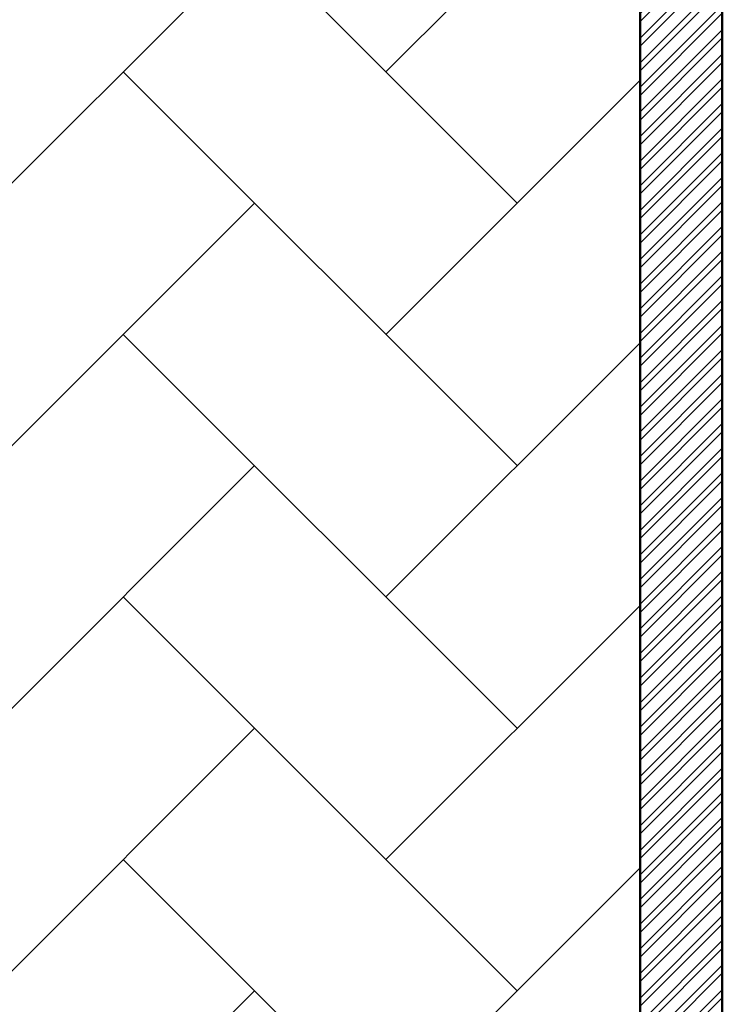
# Model space of a CAD drawing. Units: inches. Extents: x 3590 to 5167, y 65 to 1917.
# Tile 56 of 100: x 5003 to 5080, y 1450 to 1558. Entities that reach past the tile are written whole.
import ezdxf

# ---------------------------------------------------------------- set-up
doc = ezdxf.new("R2010")
doc.units = ezdxf.units.IN
for name, color, linetype, lineweight in [('A-FLOR-PATT', 8, 'Continuous', 13), ('A-WALL', 7, 'Continuous', 50), ('A-WALL-PATT', 251, 'Continuous', 13)]:
    doc.layers.add(name, color=color, linetype=linetype, lineweight=lineweight)

msp = doc.modelspace()

# ---------------------------------------------------------------- hatches: boundary and pattern name
at = {"layer": 'A-FLOR-PATT', "transparency": 33554687}
h = msp.add_hatch(dxfattribs=at)
h.set_pattern_fill('AR-HBONE', color=256, scale=0.2)
h.set_pattern_definition([(45, (-588.972, 0), (0, 28.73682), [60.96, -20.32]), (135, (-574.604, 14.368), (3e-15, 28.73682), [60.96, -20.32])])
h.paths.add_polyline_path([(5071.27, 1797), (4933.27, 1797), (4933.27, 1754), (4962.77, 1754, -0.414214), (4928.77, 1720), (4933.27, 1719), (4933.27, 1335), (5071.27, 1335)])
h.paths.add_polyline_path([(4951.78, 1521.08), (4951.72, 1521.04), (4951.56, 1520.9)], flags=16)
h.paths.add_polyline_path([(4952.27, 1521.38), (4952.2, 1521.37), (4952.2, 1521.36)], flags=0)
h.paths.add_polyline_path([(4967.05, 1529.73), (4965.23, 1528.69), (4963.41, 1527.71), (4961.76, 1526.85), (4963.59, 1527.45), (4964.04, 1527.48), (4962.98, 1527.25), (4961.76, 1526.85), (4959.79, 1525.83), (4958, 1524.89), (4956.24, 1523.93), (4954.5, 1522.92), (4954.13, 1522.68), (4953.36, 1522), (4953.37, 1522), (4953.61, 1522.06), (4955.11, 1522.76), (4956.92, 1523.43), (4958.68, 1523.92), (4960.36, 1524.2), (4961.94, 1524.29), (4964.17, 1524.11), (4965.96, 1523.31), (4963.86, 1522.98), (4965.19, 1522.5), (4963.37, 1522.5), (4961.55, 1522.49), (4959.76, 1522.46), (4958.3, 1522.42), (4957.97, 1522.39), (4956.31, 1522.23), (4954.72, 1522.07), (4953.25, 1521.9), (4953.53, 1521.62), (4954.33, 1521.38), (4956.24, 1521.23), (4958.04, 1520.93), (4959.68, 1520.48), (4961.16, 1519.9), (4963.11, 1518.8), (4964.39, 1517.33), (4962.97, 1517.73), (4964.56, 1516.66), (4965.41, 1515.71), (4963.51, 1516.32), (4961.68, 1517.01), (4959.93, 1517.74), (4958.28, 1518.53), (4956.73, 1519.34), (4955.3, 1520.17), (4954.67, 1520.57), (4954.51, 1520.63), (4955.66, 1519.32), (4956.7, 1517.98), (4957.64, 1516.65), (4958.49, 1515.33), (4959.55, 1513.52), (4960.44, 1511.77), (4958.84, 1513.62), (4957.45, 1515.32), (4955.82, 1517.46), (4956.67, 1515.45), (4957.11, 1513.92), (4957.45, 1511.71), (4957.08, 1509.79), (4956.54, 1511.11), (4955.99, 1512.57), (4955.44, 1514.13), (4954.9, 1515.74), (4954.36, 1517.36), (4953.82, 1518.94), (4953.3, 1520.45), (4953.06, 1521.12), (4952.97, 1521.15), (4952.95, 1521.09), (4952.73, 1520.2), (4953.37, 1518.02), (4953.76, 1516.37), (4954.05, 1514.77), (4954.26, 1513.22), (4954.47, 1511.13), (4954.5, 1510.4), (4954.41, 1511.76), (4954.26, 1513.22), (4954.05, 1514.77), (4953.76, 1516.37), (4953.37, 1518.02), (4952.88, 1519.7), (4952.72, 1520.14), (4952.53, 1519.06), (4952.37, 1517.79), (4952.22, 1516.31), (4952.05, 1514.6), (4951.83, 1512.63), (4951.56, 1510.36), (4951.2, 1512.17), (4950.85, 1514.34), (4950.99, 1516.38), (4951.66, 1518.29), (4952.59, 1520.48), (4952.36, 1521.13), (4951.86, 1520.33), (4950.84, 1518.91), (4949.78, 1517.59), (4948.92, 1516.62), (4948.11, 1515.26), (4947.09, 1513.55), (4945.89, 1511.61), (4946.33, 1513.4), (4946.56, 1514.25), (4945.53, 1513.33), (4944.58, 1512.53), (4946.02, 1514.51), (4947.2, 1516.05), (4947.89, 1517.31), (4949.31, 1518.76), (4950.41, 1519.77), (4950.45, 1519.81), (4952.27, 1521.38), (4951.64, 1521.49), (4950.4, 1521.18), (4948.04, 1520.36), (4946.12, 1519.45), (4944.57, 1518.47), (4943.35, 1517.44), (4942, 1515.92), (4941.66, 1515.27), (4942.81, 1516.99), (4944.57, 1518.47), (4946.12, 1519.45), (4948.04, 1520.36), (4950.4, 1521.18), (4951.64, 1521.49), (4949.65, 1521.87), (4948.6, 1521.76), (4947.13, 1521.57), (4945.42, 1521.35), (4943.45, 1521.1), (4941.18, 1520.86), (4942.86, 1521.61), (4943.87, 1522.03), (4942.95, 1521.91), (4941.41, 1521.49), (4939.54, 1520.67), (4938.97, 1520.23), (4940.73, 1521.3), (4942.95, 1521.91), (4943.7, 1522.01), (4945.89, 1522.7), (4947.56, 1522.71), (4948.92, 1522.57), (4951.13, 1522.18), (4950.97, 1522.3), (4948.13, 1523.01), (4946.03, 1523.71), (4944.23, 1524.52), (4942.71, 1525.46), (4941.44, 1526.54), (4940.43, 1527.76), (4939.65, 1529.14), (4941.42, 1528.12), (4943.15, 1527.13), (4944.84, 1526.17), (4946.51, 1525.25), (4948.18, 1524.36), (4948.36, 1524.26), (4946.48, 1526.04), (4945.18, 1527.54), (4944.19, 1529.03), (4943.5, 1530.54), (4943.28, 1531.36), (4942.5, 1531.92), (4943.11, 1531.76), (4942.96, 1533.66), (4944.14, 1531.99), (4944.61, 1531.32), (4946.2, 1530.46), (4947.49, 1529.51), (4948.79, 1528.23), (4950.37, 1526.24), (4949.49, 1528.16), (4948.85, 1530.12), (4948.49, 1532.04), (4948.38, 1533.92), (4948.5, 1535.76), (4948.83, 1537.57), (4949.42, 1535.57), (4949.96, 1533.57), (4950.46, 1531.59), (4950.96, 1529.62), (4951.39, 1527.95), (4951.72, 1530.69), (4952.2, 1532.58), (4952.89, 1534.33), (4953.77, 1535.95), (4954.83, 1537.46), (4954.52, 1535.39), (4954.27, 1533.94), (4955.58, 1535.66), (4956.75, 1536.74), (4956.16, 1534.78), (4955.59, 1532.87), (4955.04, 1531.01), (4954.52, 1529.17), (4954.04, 1527.34), (4953.64, 1525.73), (4953.61, 1525.59), (4953.4, 1524.17), (4953.38, 1524.01), (4954.07, 1525.48), (4954.91, 1527.02), (4956.14, 1528.89), (4957.85, 1530.58), (4959.38, 1531.54), (4958.26, 1530.1), (4957.14, 1528.66), (4956.07, 1527.24), (4955.06, 1525.87), (4954.14, 1524.57), (4953.35, 1523.37), (4953.31, 1523.3), (4953.27, 1522.92), (4953.26, 1522.38), (4954.1, 1523.37), (4954.63, 1524.28), (4955.96, 1526.36), (4957.23, 1528.13), (4958.42, 1529.61), (4960.04, 1531.37), (4961.37, 1532.38), (4962.1, 1532.77), (4961.07, 1531.06), (4959.99, 1529.44), (4958.87, 1527.91), (4958.15, 1527.01), (4959.8, 1528), (4961.59, 1528.79), (4963.39, 1529.33), (4965.21, 1529.63)], flags=16)
h.paths.add_polyline_path([(4962.94, 1523.18), (4961.11, 1523.42), (4960.39, 1523.36), (4962.35, 1523.33)], flags=0)
h.paths.add_polyline_path([(5049.54, 1584.55), (5049.48, 1584.51), (5049.32, 1584.37)], flags=16)
h.paths.add_polyline_path([(5050.03, 1584.85), (5049.96, 1584.85), (5049.96, 1584.83)], flags=0)
h.paths.add_polyline_path([(5042.33, 1581.95), (5043.88, 1582.93), (5045.81, 1583.83), (5048.16, 1584.65), (5049.41, 1584.97), (5047.41, 1585.34), (5046.36, 1585.23), (5044.89, 1585.04), (5043.18, 1584.82), (5041.21, 1584.58), (5038.94, 1584.33), (5040.62, 1585.09), (5041.63, 1585.5), (5040.71, 1585.38), (5039.17, 1584.96), (5037.3, 1584.14), (5036.73, 1583.7), (5038.49, 1584.77), (5040.71, 1585.38), (5041.46, 1585.48), (5043.66, 1586.17), (5045.33, 1586.19), (5046.68, 1586.04), (5048.89, 1585.66), (5048.73, 1585.77), (5045.89, 1586.48), (5043.8, 1587.18), (5041.99, 1588), (5040.47, 1588.94), (5039.21, 1590.01), (5038.19, 1591.23), (5037.41, 1592.62), (5039.18, 1591.6), (5040.91, 1590.61), (5042.6, 1589.65), (5044.28, 1588.72), (5045.94, 1587.83), (5046.13, 1587.74), (5044.24, 1589.52), (5042.94, 1591.01), (5041.95, 1592.51), (5041.26, 1594.01), (5041.04, 1594.83), (5040.26, 1595.39), (5040.87, 1595.24), (5040.72, 1597.13), (5041.9, 1595.46), (5042.37, 1594.8), (5043.96, 1593.94), (5045.25, 1592.98), (5046.55, 1591.7), (5048.13, 1589.71), (5047.25, 1591.63), (5046.61, 1593.6), (5046.25, 1595.52), (5046.14, 1597.39), (5046.26, 1599.23), (5046.59, 1601.05), (5047.18, 1599.04), (5047.72, 1597.04), (5048.23, 1595.06), (5048.72, 1593.09), (5049.15, 1591.43), (5049.48, 1594.16), (5049.96, 1596.05), (5050.65, 1597.8), (5051.53, 1599.43), (5052.59, 1600.93), (5052.28, 1598.86), (5052.03, 1597.41), (5053.34, 1599.14), (5054.51, 1600.21), (5053.92, 1598.25), (5053.35, 1596.35), (5052.8, 1594.48), (5052.29, 1592.64), (5051.8, 1590.82), (5051.4, 1589.21), (5051.37, 1589.06), (5051.16, 1587.64), (5051.14, 1587.48), (5051.83, 1588.95), (5052.67, 1590.5), (5053.9, 1592.37), (5055.61, 1594.05), (5057.14, 1595.01), (5056.02, 1593.58), (5054.9, 1592.14), (5053.83, 1590.72), (5052.82, 1589.34), (5051.9, 1588.05), (5051.11, 1586.85), (5051.07, 1586.78), (5051.03, 1586.4), (5051.02, 1585.86), (5051.86, 1586.85), (5052.39, 1587.76), (5053.72, 1589.83), (5054.99, 1591.6), (5056.18, 1593.08), (5057.8, 1594.84), (5059.13, 1595.85), (5059.86, 1596.24), (5058.83, 1594.54), (5057.75, 1592.91), (5056.63, 1591.38), (5055.91, 1590.48), (5057.56, 1591.48), (5059.35, 1592.27), (5061.15, 1592.8), (5062.97, 1593.11), (5064.81, 1593.2), (5062.99, 1592.17), (5061.17, 1591.19), (5059.52, 1590.32), (5061.35, 1590.92), (5061.8, 1590.95), (5060.74, 1590.72), (5059.52, 1590.33), (5057.55, 1589.31), (5055.77, 1588.37), (5054, 1587.4), (5052.27, 1586.39), (5051.89, 1586.16), (5051.12, 1585.47), (5051.13, 1585.47), (5051.37, 1585.54), (5052.87, 1586.24), (5054.68, 1586.91), (5056.44, 1587.39), (5058.12, 1587.67), (5059.71, 1587.76), (5061.93, 1587.58), (5063.72, 1586.78), (5061.62, 1586.45), (5062.95, 1585.97), (5061.13, 1585.97), (5059.31, 1585.96), (5057.52, 1585.93), (5056.07, 1585.89), (5055.73, 1585.86), (5054.07, 1585.71), (5052.48, 1585.55), (5051.01, 1585.37), (5051.29, 1585.1), (5052.09, 1584.85), (5054, 1584.7), (5055.8, 1584.4), (5057.45, 1583.96), (5058.92, 1583.37), (5060.87, 1582.27), (5062.15, 1580.8), (5060.73, 1581.2), (5062.32, 1580.13), (5063.17, 1579.18), (5061.27, 1579.8), (5059.44, 1580.48), (5057.7, 1581.22), (5056.04, 1582), (5054.49, 1582.82), (5053.06, 1583.65), (5052.43, 1584.05), (5052.27, 1584.1), (5053.42, 1582.79), (5054.46, 1581.46), (5055.41, 1580.12), (5056.25, 1578.81), (5057.31, 1577), (5058.2, 1575.24), (5056.6, 1577.09), (5055.21, 1578.8), (5053.58, 1580.93), (5054.43, 1578.92), (5054.87, 1577.4), (5055.21, 1575.19), (5054.84, 1573.27), (5054.3, 1574.58), (5053.75, 1576.04), (5053.21, 1577.6), (5052.66, 1579.21), (5052.12, 1580.83), (5051.59, 1582.42), (5051.07, 1583.93), (5050.83, 1584.59), (5050.73, 1584.62), (5050.71, 1584.56), (5050.49, 1583.67), (5051.13, 1581.5), (5051.52, 1579.85), (5051.81, 1578.24), (5052.03, 1576.7), (5052.23, 1574.61), (5052.26, 1573.88), (5052.17, 1575.23), (5052.03, 1576.7), (5051.81, 1578.24), (5051.52, 1579.85), (5051.13, 1581.5), (5050.64, 1583.17), (5050.48, 1583.62), (5050.29, 1582.53), (5050.14, 1581.26), (5049.98, 1579.79), (5049.81, 1578.07), (5049.59, 1576.1), (5049.32, 1573.84), (5048.96, 1575.64), (5048.61, 1577.81), (5048.75, 1579.85), (5049.42, 1581.76), (5050.35, 1583.96), (5050.12, 1584.6), (5049.62, 1583.8), (5048.6, 1582.38), (5047.54, 1581.06), (5046.68, 1580.09), (5045.87, 1578.73), (5044.85, 1577.03), (5043.65, 1575.09), (5044.09, 1576.88), (5044.32, 1577.72), (5043.29, 1576.8), (5042.34, 1576.01), (5043.78, 1577.98), (5044.97, 1579.52), (5045.65, 1580.79), (5047.07, 1582.24), (5048.18, 1583.24), (5048.21, 1583.28), (5050.03, 1584.85), (5049.41, 1584.97), (5048.16, 1584.65), (5045.81, 1583.83), (5043.88, 1582.93), (5042.33, 1581.95), (5041.11, 1580.92), (5039.76, 1579.39), (5039.42, 1578.75), (5040.57, 1580.46)], flags=16)
h.paths.add_polyline_path([(4954.8, 1533.12), (4954.26, 1532.08), (4953.83, 1530.93), (4953.5, 1529.64), (4953.28, 1528.13), (4953.17, 1526.38), (4953.16, 1524.32), (4953.28, 1521.24), (4952.8, 1521.84), (4951.56, 1522), (4950.98, 1521.96), (4952.66, 1521.94), (4952.8, 1521.84), (4953.15, 1523.59), (4953.17, 1526.38), (4953.28, 1528.13), (4953.61, 1530.35), (4954.46, 1532.59)], flags=0)
h.paths.add_polyline_path([(5050.56, 1585.32), (5049.32, 1585.47), (5048.74, 1585.44), (5050.42, 1585.42), (5050.56, 1585.32), (5050.91, 1587.07), (5050.93, 1589.85), (5051.04, 1591.61), (5051.37, 1593.82), (5052.22, 1596.07), (5052.56, 1596.59), (5052.02, 1595.55), (5051.59, 1594.41), (5051.27, 1593.11), (5051.04, 1591.61), (5050.93, 1589.85), (5050.92, 1587.79), (5051.04, 1584.71)], flags=0)
h.paths.add_polyline_path([(5058.15, 1586.84), (5060.11, 1586.8), (5060.71, 1586.66), (5058.87, 1586.9)], flags=0)
h.paths.add_polyline_path([(5049.54, 1430.94), (5049.48, 1430.9), (5049.32, 1430.75)], flags=16)
h.paths.add_polyline_path([(5050.03, 1431.24), (5049.96, 1431.23), (5049.96, 1431.21)], flags=0)
h.paths.add_polyline_path([(5046.59, 1447.43), (5047.18, 1445.42), (5047.72, 1443.43), (5048.23, 1441.45), (5048.72, 1439.48), (5049.15, 1437.81), (5049.48, 1440.55), (5049.96, 1442.44), (5050.65, 1444.19), (5051.53, 1445.81), (5052.59, 1447.32), (5052.28, 1445.25), (5052.03, 1443.8), (5053.34, 1445.52), (5054.51, 1446.6), (5053.92, 1444.64), (5053.35, 1442.73), (5052.8, 1440.87), (5052.29, 1439.03), (5051.8, 1437.2), (5051.4, 1435.59), (5051.37, 1435.45), (5051.16, 1434.03), (5051.14, 1433.87), (5051.83, 1435.34), (5052.67, 1436.88), (5053.9, 1438.75), (5055.61, 1440.44), (5057.14, 1441.4), (5056.02, 1439.96), (5054.9, 1438.52), (5053.83, 1437.1), (5052.82, 1435.73), (5051.9, 1434.43), (5051.11, 1433.23), (5051.07, 1433.16), (5051.03, 1432.78), (5051.02, 1432.24), (5051.86, 1433.23), (5052.39, 1434.14), (5053.72, 1436.22), (5054.99, 1437.99), (5056.18, 1439.47), (5057.8, 1441.23), (5059.13, 1442.23), (5059.86, 1442.63), (5058.83, 1440.92), (5057.75, 1439.3), (5056.63, 1437.77), (5055.91, 1436.87), (5057.56, 1437.86), (5059.35, 1438.65), (5061.15, 1439.19), (5062.97, 1439.49), (5064.81, 1439.59), (5062.99, 1438.55), (5061.17, 1437.57), (5059.52, 1436.71), (5061.35, 1437.31), (5061.8, 1437.34), (5060.74, 1437.11), (5059.52, 1436.71), (5057.55, 1435.69), (5055.77, 1434.75), (5054, 1433.79), (5052.27, 1432.78), (5051.89, 1432.54), (5051.12, 1431.86), (5051.13, 1431.86), (5051.37, 1431.92), (5052.87, 1432.62), (5054.68, 1433.29), (5056.44, 1433.77), (5058.12, 1434.06), (5059.71, 1434.15), (5061.93, 1433.97), (5063.72, 1433.17), (5061.62, 1432.84), (5062.95, 1432.36), (5061.13, 1432.36), (5059.31, 1432.35), (5057.52, 1432.32), (5056.07, 1432.28), (5055.73, 1432.25), (5054.07, 1432.09), (5052.48, 1431.93), (5051.01, 1431.76), (5051.29, 1431.48), (5052.09, 1431.24), (5054, 1431.09), (5055.8, 1430.79), (5057.45, 1430.34), (5058.92, 1429.76), (5060.87, 1428.66), (5062.15, 1427.18), (5060.73, 1427.59), (5062.32, 1426.52), (5063.17, 1425.57), (5061.27, 1426.18), (5059.44, 1426.86), (5057.7, 1427.6), (5056.04, 1428.39), (5054.49, 1429.2), (5053.06, 1430.03), (5052.43, 1430.43), (5052.27, 1430.49), (5053.42, 1429.18), (5054.46, 1427.84), (5055.41, 1426.51), (5056.25, 1425.19), (5057.31, 1423.38), (5058.2, 1421.63), (5056.6, 1423.48), (5055.21, 1425.18), (5053.58, 1427.32), (5054.43, 1425.31), (5054.87, 1423.78), (5055.21, 1421.57), (5054.84, 1419.65), (5054.3, 1420.97), (5053.75, 1422.43), (5053.21, 1423.98), (5052.66, 1425.59), (5052.12, 1427.21), (5051.59, 1428.8), (5051.07, 1430.31), (5050.83, 1430.98), (5050.73, 1431.01), (5050.71, 1430.95), (5050.49, 1430.06), (5051.13, 1427.88), (5051.52, 1426.23), (5051.81, 1424.62), (5052.03, 1423.08), (5052.23, 1420.99), (5052.26, 1420.26), (5052.17, 1421.62), (5052.03, 1423.08), (5051.81, 1424.62), (5051.52, 1426.23), (5051.13, 1427.88), (5050.64, 1429.56), (5050.48, 1430), (5050.29, 1428.92), (5050.14, 1427.65), (5049.98, 1426.17), (5049.81, 1424.46), (5049.59, 1422.49), (5049.32, 1420.22), (5048.96, 1422.03), (5048.61, 1424.2), (5048.75, 1426.24), (5049.42, 1428.15), (5050.35, 1430.34), (5050.12, 1430.99), (5049.62, 1430.19), (5048.6, 1428.77), (5047.54, 1427.45), (5046.68, 1426.48), (5045.87, 1425.12), (5044.85, 1423.41), (5043.65, 1421.47), (5044.09, 1423.26), (5044.32, 1424.11), (5043.29, 1423.19), (5042.34, 1422.39), (5043.78, 1424.37), (5044.97, 1425.91), (5045.65, 1427.17), (5047.07, 1428.62), (5048.18, 1429.63), (5048.21, 1429.67), (5050.03, 1431.24), (5049.41, 1431.35), (5048.16, 1431.04), (5045.81, 1430.22), (5043.88, 1429.31), (5042.33, 1428.33), (5041.11, 1427.3), (5039.76, 1425.78), (5039.42, 1425.13), (5040.57, 1426.85), (5042.33, 1428.33), (5043.88, 1429.31), (5045.81, 1430.22), (5048.16, 1431.04), (5049.41, 1431.35), (5047.41, 1431.73), (5046.36, 1431.62), (5044.89, 1431.43), (5043.18, 1431.21), (5041.21, 1430.96), (5038.94, 1430.72), (5040.62, 1431.47), (5041.63, 1431.89), (5040.71, 1431.77), (5039.17, 1431.34), (5037.3, 1430.53), (5036.73, 1430.08), (5038.49, 1431.16), (5040.71, 1431.77), (5041.46, 1431.87), (5043.66, 1432.56), (5045.33, 1432.57), (5046.68, 1432.43), (5048.89, 1432.04), (5048.73, 1432.16), (5045.89, 1432.87), (5043.8, 1433.57), (5041.99, 1434.38), (5040.47, 1435.32), (5039.21, 1436.4), (5038.19, 1437.62), (5037.41, 1439), (5039.18, 1437.98), (5040.91, 1436.99), (5042.6, 1436.03), (5044.28, 1435.11), (5045.94, 1434.22), (5046.13, 1434.12), (5044.24, 1435.9), (5042.94, 1437.4), (5041.95, 1438.89), (5041.26, 1440.4), (5041.04, 1441.22), (5040.26, 1441.78), (5040.87, 1441.62), (5040.72, 1443.52), (5041.9, 1441.85), (5042.37, 1441.18), (5043.96, 1440.32), (5045.25, 1439.37), (5046.55, 1438.09), (5048.13, 1436.1), (5047.25, 1438.01), (5046.61, 1439.98), (5046.25, 1441.9), (5046.14, 1443.78), (5046.26, 1445.62)], flags=16)
h.paths.add_polyline_path([(5052.38, 1444.25), (5051.62, 1442.78), (5052.02, 1441.94), (5052.56, 1442.98)], flags=0)
h.paths.add_polyline_path([(5050.56, 1431.7), (5049.32, 1431.86), (5048.74, 1431.82), (5050.42, 1431.8)], flags=0)
h.paths.add_polyline_path([(5058.15, 1433.22), (5060.11, 1433.19), (5060.71, 1433.04), (5058.87, 1433.28)], flags=0)
h.paths.add_polyline_path([(5049.54, 1352.29), (5049.48, 1352.25), (5049.32, 1352.1)], flags=16)
h.paths.add_polyline_path([(5050.03, 1352.59), (5049.96, 1352.58), (5049.96, 1352.56)], flags=0)
h.paths.add_polyline_path([(5046.59, 1368.78), (5047.18, 1366.77), (5047.72, 1364.78), (5048.23, 1362.79), (5048.72, 1360.83), (5049.15, 1359.16), (5049.48, 1361.9), (5049.96, 1363.79), (5050.65, 1365.54), (5051.53, 1367.16), (5052.59, 1368.67), (5052.28, 1366.6), (5052.03, 1365.15), (5053.34, 1366.87), (5054.51, 1367.95), (5053.92, 1365.99), (5053.35, 1364.08), (5052.8, 1362.21), (5052.29, 1360.37), (5051.8, 1358.55), (5051.4, 1356.94), (5051.37, 1356.79), (5051.16, 1355.37), (5051.14, 1355.22), (5051.83, 1356.68), (5052.67, 1358.23), (5053.9, 1360.1), (5055.61, 1361.79), (5057.14, 1362.75), (5056.02, 1361.31), (5054.9, 1359.87), (5053.83, 1358.45), (5052.82, 1357.08), (5051.9, 1355.78), (5051.11, 1354.58), (5051.07, 1354.51), (5051.03, 1354.13), (5051.02, 1353.59), (5051.86, 1354.58), (5052.39, 1355.49), (5053.72, 1357.57), (5054.99, 1359.34), (5056.18, 1360.82), (5057.8, 1362.58), (5059.13, 1363.58), (5059.86, 1363.98), (5058.83, 1362.27), (5057.75, 1360.65), (5056.63, 1359.12), (5055.91, 1358.22), (5057.56, 1359.21), (5059.35, 1360), (5061.15, 1360.54), (5062.97, 1360.84), (5064.81, 1360.94), (5062.99, 1359.9), (5061.17, 1358.92), (5059.52, 1358.06), (5061.35, 1358.66), (5061.8, 1358.69), (5060.74, 1358.46), (5059.52, 1358.06), (5057.55, 1357.04), (5055.77, 1356.1), (5054, 1355.14), (5052.27, 1354.13), (5051.89, 1353.89), (5051.12, 1353.21), (5051.13, 1353.21), (5051.37, 1353.27), (5052.87, 1353.97), (5054.68, 1354.64), (5056.44, 1355.12), (5058.12, 1355.41), (5059.71, 1355.49), (5061.93, 1355.32), (5063.72, 1354.52), (5061.62, 1354.18), (5062.95, 1353.71), (5061.13, 1353.71), (5059.31, 1353.7), (5057.52, 1353.67), (5056.07, 1353.63), (5055.73, 1353.6), (5054.07, 1353.44), (5052.48, 1353.28), (5051.01, 1353.11), (5051.29, 1352.83), (5052.09, 1352.59), (5054, 1352.44), (5055.8, 1352.14), (5057.45, 1351.69), (5058.92, 1351.1), (5060.87, 1350.01), (5062.15, 1348.53), (5060.73, 1348.93), (5062.32, 1347.87), (5063.17, 1346.92), (5061.27, 1347.53), (5059.44, 1348.21), (5057.7, 1348.95), (5056.04, 1349.74), (5054.49, 1350.55), (5053.06, 1351.38), (5052.43, 1351.78), (5052.27, 1351.84), (5053.42, 1350.53), (5054.46, 1349.19), (5055.41, 1347.86), (5056.25, 1346.54), (5057.31, 1344.73), (5058.2, 1342.98), (5056.6, 1344.83), (5055.21, 1346.53), (5053.58, 1348.67), (5054.43, 1346.66), (5054.87, 1345.13), (5055.21, 1342.92), (5054.84, 1341), (5054.3, 1342.32), (5053.75, 1343.78), (5053.21, 1345.33), (5052.66, 1346.94), (5052.12, 1348.56), (5051.59, 1350.15), (5051.07, 1351.66), (5050.83, 1352.32), (5050.73, 1352.35), (5050.71, 1352.3), (5050.49, 1351.41), (5051.13, 1349.23), (5051.52, 1347.58), (5051.81, 1345.97), (5052.03, 1344.43), (5052.23, 1342.34), (5052.26, 1341.61), (5052.17, 1342.97), (5052.03, 1344.43), (5051.81, 1345.97), (5051.52, 1347.58), (5051.13, 1349.23), (5050.64, 1350.91), (5050.48, 1351.35), (5050.29, 1350.27), (5050.14, 1349), (5049.98, 1347.52), (5049.81, 1345.81), (5049.59, 1343.83), (5049.32, 1341.57), (5048.96, 1343.38), (5048.61, 1345.55), (5048.75, 1347.58), (5049.42, 1349.49), (5050.35, 1351.69), (5050.12, 1352.34), (5049.62, 1351.54), (5048.6, 1350.12), (5047.54, 1348.8), (5046.68, 1347.83), (5045.87, 1346.46), (5044.85, 1344.76), (5043.65, 1342.82), (5044.09, 1344.61), (5044.32, 1345.46), (5043.29, 1344.54), (5042.34, 1343.74), (5043.78, 1345.72), (5044.97, 1347.26), (5045.65, 1348.52), (5047.07, 1349.97), (5048.18, 1350.98), (5048.21, 1351.01), (5050.03, 1352.59), (5049.41, 1352.7), (5048.16, 1352.39), (5045.81, 1351.57), (5043.88, 1350.66), (5042.33, 1349.68), (5041.11, 1348.65), (5039.76, 1347.13), (5039.42, 1346.48), (5040.57, 1348.2), (5042.33, 1349.68), (5043.88, 1350.66), (5045.81, 1351.57), (5048.16, 1352.39), (5049.41, 1352.7), (5047.41, 1353.08), (5046.36, 1352.96), (5044.89, 1352.78), (5043.18, 1352.56), (5041.21, 1352.31), (5038.94, 1352.06), (5040.62, 1352.82), (5041.63, 1353.24), (5040.71, 1353.12), (5039.17, 1352.69), (5037.3, 1351.88), (5036.73, 1351.43), (5038.49, 1352.51), (5040.71, 1353.12), (5041.46, 1353.22), (5043.66, 1353.91), (5045.33, 1353.92), (5046.68, 1353.77), (5048.89, 1353.39), (5048.73, 1353.51), (5045.89, 1354.21), (5043.8, 1354.92), (5041.99, 1355.73), (5040.47, 1356.67), (5039.21, 1357.75), (5038.19, 1358.97), (5037.41, 1360.35), (5039.18, 1359.33), (5040.91, 1358.34), (5042.6, 1357.38), (5044.28, 1356.46), (5045.94, 1355.57), (5046.13, 1355.47), (5044.24, 1357.25), (5042.94, 1358.75), (5041.95, 1360.24), (5041.26, 1361.75), (5041.04, 1362.57), (5040.26, 1363.13), (5040.87, 1362.97), (5040.72, 1364.87), (5041.9, 1363.2), (5042.37, 1362.53), (5043.96, 1361.67), (5045.25, 1360.72), (5046.55, 1359.44), (5048.13, 1357.45), (5047.25, 1359.36), (5046.61, 1361.33), (5046.25, 1363.25), (5046.14, 1365.13), (5046.26, 1366.97)], flags=16)
h.paths.add_polyline_path([(5052.38, 1365.6), (5051.62, 1364.13), (5052.02, 1363.29), (5052.56, 1364.33)], flags=0)
h.paths.add_polyline_path([(4951.78, 1698.04), (4951.72, 1698), (4951.56, 1697.86)], flags=16)
h.paths.add_polyline_path([(4952.27, 1698.34), (4952.2, 1698.34), (4952.2, 1698.32)], flags=0)
h.paths.add_polyline_path([(4957.08, 1686.76), (4956.54, 1688.07), (4955.99, 1689.53), (4955.44, 1691.09), (4954.9, 1692.7), (4954.36, 1694.32), (4953.82, 1695.91), (4953.3, 1697.42), (4953.06, 1698.08), (4952.97, 1698.11), (4952.95, 1698.05), (4952.73, 1697.16), (4953.37, 1694.99), (4953.76, 1693.34), (4954.05, 1691.73), (4954.26, 1690.19), (4954.47, 1688.1), (4954.5, 1687.37), (4954.41, 1688.72), (4954.26, 1690.19), (4954.05, 1691.73), (4953.76, 1693.34), (4953.37, 1694.99), (4952.88, 1696.66), (4952.72, 1697.11), (4952.53, 1696.02), (4952.37, 1694.75), (4952.22, 1693.28), (4952.05, 1691.56), (4951.83, 1689.59), (4951.56, 1687.33), (4951.2, 1689.13), (4950.85, 1691.3), (4950.99, 1693.34), (4951.66, 1695.25), (4952.59, 1697.44), (4952.36, 1698.09), (4951.86, 1697.29), (4950.84, 1695.87), (4949.78, 1694.55), (4948.92, 1693.58), (4948.11, 1692.22), (4947.09, 1690.52), (4945.89, 1688.58), (4946.33, 1690.37), (4946.56, 1691.21), (4945.53, 1690.29), (4944.58, 1689.5), (4946.02, 1691.47), (4947.2, 1693.01), (4947.89, 1694.28), (4949.31, 1695.73), (4950.41, 1696.73), (4950.45, 1696.77), (4952.27, 1698.34), (4951.64, 1698.46), (4950.4, 1698.14), (4948.04, 1697.32), (4946.12, 1696.42), (4944.57, 1695.44), (4943.35, 1694.41), (4942, 1692.88), (4941.66, 1692.24), (4942.81, 1693.95), (4944.57, 1695.44), (4946.12, 1696.42), (4948.04, 1697.32), (4950.4, 1698.14), (4951.64, 1698.46), (4949.65, 1698.83), (4948.6, 1698.72), (4947.13, 1698.53), (4945.42, 1698.31), (4943.45, 1698.07), (4941.18, 1697.82), (4942.86, 1698.58), (4943.87, 1698.99), (4942.95, 1698.87), (4941.41, 1698.45), (4939.54, 1697.63), (4938.97, 1697.19), (4940.73, 1698.26), (4942.95, 1698.87), (4943.7, 1698.97), (4945.89, 1699.66), (4947.56, 1699.68), (4948.92, 1699.53), (4951.13, 1699.15), (4950.97, 1699.26), (4948.13, 1699.97), (4946.03, 1700.67), (4944.23, 1701.49), (4942.71, 1702.43), (4941.44, 1703.5), (4940.43, 1704.72), (4939.65, 1706.11), (4941.42, 1705.09), (4943.15, 1704.1), (4944.84, 1703.14), (4946.51, 1702.21), (4948.18, 1701.32), (4948.36, 1701.23), (4946.48, 1703.01), (4945.18, 1704.5), (4944.19, 1706), (4943.5, 1707.5), (4943.28, 1708.32), (4942.5, 1708.88), (4943.11, 1708.73), (4942.96, 1710.62), (4944.14, 1708.95), (4944.61, 1708.29), (4946.2, 1707.43), (4947.49, 1706.47), (4948.79, 1705.19), (4950.37, 1703.2), (4949.49, 1705.12), (4948.85, 1707.09), (4948.49, 1709.01), (4948.38, 1710.88), (4948.5, 1712.72), (4948.83, 1714.54), (4949.42, 1712.53), (4949.96, 1710.53), (4950.46, 1708.55), (4950.96, 1706.58), (4951.39, 1704.92), (4951.72, 1707.65), (4952.2, 1709.54), (4952.89, 1711.29), (4953.77, 1712.92), (4954.83, 1714.42), (4954.52, 1712.35), (4954.27, 1710.9), (4955.58, 1712.63), (4956.75, 1713.7), (4956.16, 1711.74), (4955.59, 1709.84), (4955.04, 1707.97), (4954.52, 1706.13), (4954.04, 1704.31), (4953.64, 1702.7), (4953.61, 1702.55), (4953.4, 1701.13), (4953.38, 1700.97), (4954.07, 1702.44), (4954.91, 1703.99), (4956.14, 1705.86), (4957.85, 1707.54), (4959.38, 1708.5), (4958.26, 1707.07), (4957.14, 1705.63), (4956.07, 1704.21), (4955.06, 1702.83), (4954.14, 1701.54), (4953.35, 1700.34), (4953.31, 1700.27), (4953.27, 1699.89), (4953.26, 1699.35), (4954.1, 1700.34), (4954.63, 1701.25), (4955.96, 1703.32), (4957.23, 1705.09), (4958.42, 1706.57), (4960.04, 1708.33), (4961.37, 1709.34), (4962.1, 1709.73), (4961.07, 1708.03), (4959.99, 1706.4), (4958.87, 1704.87), (4958.15, 1703.97), (4959.8, 1704.97), (4961.59, 1705.76), (4963.39, 1706.29), (4965.21, 1706.6), (4967.05, 1706.69), (4965.23, 1705.66), (4963.41, 1704.68), (4961.76, 1703.81), (4963.59, 1704.41), (4964.04, 1704.44), (4962.98, 1704.21), (4961.76, 1703.82), (4959.79, 1702.8), (4958, 1701.86), (4956.24, 1700.89), (4954.5, 1699.88), (4954.13, 1699.65), (4953.36, 1698.96), (4953.37, 1698.96), (4953.61, 1699.03), (4955.11, 1699.72), (4956.92, 1700.4), (4958.68, 1700.88), (4960.36, 1701.16), (4961.94, 1701.25), (4964.17, 1701.07), (4965.96, 1700.27), (4963.86, 1699.94), (4965.19, 1699.46), (4963.37, 1699.46), (4961.55, 1699.45), (4959.76, 1699.42), (4958.3, 1699.38), (4957.97, 1699.35), (4956.31, 1699.2), (4954.72, 1699.04), (4953.25, 1698.86), (4953.53, 1698.59), (4954.33, 1698.34), (4956.24, 1698.19), (4958.04, 1697.89), (4959.68, 1697.45), (4961.16, 1696.86), (4963.11, 1695.76), (4964.39, 1694.29), (4962.97, 1694.69), (4964.56, 1693.62), (4965.41, 1692.67), (4963.51, 1693.29), (4961.68, 1693.97), (4959.93, 1694.71), (4958.28, 1695.49), (4956.73, 1696.31), (4955.3, 1697.14), (4954.67, 1697.54), (4954.51, 1697.59), (4955.66, 1696.28), (4956.7, 1694.95), (4957.64, 1693.61), (4958.49, 1692.3), (4959.55, 1690.49), (4960.44, 1688.73), (4958.84, 1690.58), (4957.45, 1692.29), (4955.82, 1694.42), (4956.67, 1692.41), (4957.11, 1690.89), (4957.45, 1688.68)], flags=16)
h.paths.add_polyline_path([(5050.56, 1353.05), (5049.32, 1353.21), (5048.74, 1353.17), (5050.42, 1353.15)], flags=0)
h.paths.add_polyline_path([(4951.78, 1351.49), (4951.72, 1351.45), (4951.56, 1351.3)], flags=16)
h.paths.add_polyline_path([(4952.27, 1351.79), (4952.2, 1351.78), (4952.2, 1351.76)], flags=0)
h.paths.add_polyline_path([(4954.83, 1367.87), (4954.52, 1365.8), (4954.27, 1364.35), (4955.58, 1366.07), (4956.75, 1367.15), (4956.16, 1365.19), (4955.59, 1363.28), (4955.04, 1361.42), (4954.52, 1359.58), (4954.04, 1357.75), (4953.64, 1356.14), (4953.61, 1356), (4953.4, 1354.58), (4953.38, 1354.42), (4954.07, 1355.89), (4954.91, 1357.43), (4956.14, 1359.3), (4957.85, 1360.99), (4959.38, 1361.95), (4958.26, 1360.51), (4957.14, 1359.07), (4956.07, 1357.65), (4955.06, 1356.28), (4954.14, 1354.98), (4953.35, 1353.78), (4953.31, 1353.71), (4953.27, 1353.33), (4953.26, 1352.79), (4954.1, 1353.78), (4954.63, 1354.69), (4955.96, 1356.77), (4957.23, 1358.54), (4958.42, 1360.02), (4960.04, 1361.78), (4961.37, 1362.78), (4962.1, 1363.18), (4961.07, 1361.47), (4959.99, 1359.85), (4958.87, 1358.32), (4958.15, 1357.42), (4959.8, 1358.41), (4961.59, 1359.2), (4963.39, 1359.74), (4965.21, 1360.04), (4967.05, 1360.14), (4965.23, 1359.1), (4963.41, 1358.12), (4961.76, 1357.26), (4963.59, 1357.86), (4964.04, 1357.89), (4962.98, 1357.66), (4961.76, 1357.26), (4959.79, 1356.24), (4958, 1355.3), (4956.24, 1354.34), (4954.5, 1353.33), (4954.13, 1353.09), (4953.36, 1352.41), (4953.37, 1352.41), (4953.61, 1352.47), (4955.11, 1353.17), (4956.92, 1353.84), (4958.68, 1354.32), (4960.36, 1354.61), (4961.94, 1354.7), (4964.17, 1354.52), (4965.96, 1353.72), (4963.86, 1353.39), (4965.19, 1352.91), (4963.37, 1352.91), (4961.55, 1352.9), (4959.76, 1352.87), (4958.3, 1352.83), (4957.97, 1352.8), (4956.31, 1352.64), (4954.72, 1352.48), (4953.25, 1352.31), (4953.53, 1352.03), (4954.33, 1351.79), (4956.24, 1351.64), (4958.04, 1351.34), (4959.68, 1350.89), (4961.16, 1350.31), (4963.11, 1349.21), (4964.39, 1347.73), (4962.97, 1348.14), (4964.56, 1347.07), (4965.41, 1346.12), (4963.51, 1346.73), (4961.68, 1347.41), (4959.93, 1348.15), (4958.28, 1348.94), (4956.73, 1349.75), (4955.3, 1350.58), (4954.67, 1350.98), (4954.51, 1351.04), (4955.66, 1349.73), (4956.7, 1348.39), (4957.64, 1347.06), (4958.49, 1345.74), (4959.55, 1343.93), (4960.44, 1342.18), (4958.84, 1344.03), (4957.45, 1345.73), (4955.82, 1347.87), (4956.67, 1345.86), (4957.11, 1344.33), (4957.45, 1342.12), (4957.08, 1340.2), (4956.54, 1341.52), (4955.99, 1342.98), (4955.44, 1344.53), (4954.9, 1346.14), (4954.36, 1347.76), (4953.82, 1349.35), (4953.3, 1350.86), (4953.06, 1351.53), (4952.97, 1351.56), (4952.95, 1351.5), (4952.73, 1350.61), (4953.37, 1348.43), (4953.76, 1346.78), (4954.05, 1345.17), (4954.26, 1343.63), (4954.47, 1341.54), (4954.5, 1340.81), (4954.41, 1342.17), (4954.26, 1343.63), (4954.05, 1345.17), (4953.76, 1346.78), (4953.37, 1348.43), (4952.88, 1350.11), (4952.72, 1350.55), (4952.53, 1349.47), (4952.37, 1348.2), (4952.22, 1346.72), (4952.05, 1345.01), (4951.83, 1343.04), (4951.56, 1340.77), (4951.2, 1342.58), (4950.85, 1344.75), (4950.99, 1346.79), (4951.66, 1348.7), (4952.59, 1350.89), (4952.36, 1351.54), (4951.86, 1350.74), (4950.84, 1349.32), (4949.78, 1348), (4948.92, 1347.03), (4948.11, 1345.67), (4947.09, 1343.96), (4945.89, 1342.02), (4946.33, 1343.81), (4946.56, 1344.66), (4945.53, 1343.74), (4944.58, 1342.94), (4946.02, 1344.92), (4947.2, 1346.46), (4947.89, 1347.72), (4949.31, 1349.17), (4950.41, 1350.18), (4950.45, 1350.22), (4952.27, 1351.79), (4951.64, 1351.9), (4950.4, 1351.59), (4948.04, 1350.77), (4946.12, 1349.86), (4944.57, 1348.88), (4943.35, 1347.85), (4942, 1346.33), (4941.66, 1345.68), (4942.81, 1347.4), (4944.57, 1348.88), (4946.12, 1349.86), (4948.04, 1350.77), (4950.4, 1351.59), (4951.64, 1351.9), (4949.65, 1352.28), (4948.6, 1352.17), (4947.13, 1351.98), (4945.42, 1351.76), (4943.45, 1351.51), (4941.18, 1351.27), (4942.86, 1352.02), (4943.87, 1352.44), (4942.95, 1352.32), (4941.41, 1351.89), (4939.54, 1351.08), (4938.97, 1350.63), (4940.73, 1351.71), (4942.95, 1352.32), (4943.7, 1352.42), (4945.89, 1353.11), (4947.56, 1353.12), (4948.92, 1352.98), (4951.13, 1352.59), (4950.97, 1352.71), (4948.13, 1353.42), (4946.03, 1354.12), (4944.23, 1354.93), (4942.71, 1355.87), (4941.44, 1356.95), (4940.43, 1358.17), (4939.65, 1359.55), (4941.42, 1358.53), (4943.15, 1357.54), (4944.84, 1356.58), (4946.51, 1355.66), (4948.18, 1354.77), (4948.36, 1354.67), (4946.48, 1356.45), (4945.18, 1357.95), (4944.19, 1359.44), (4943.5, 1360.95), (4943.28, 1361.77), (4942.5, 1362.33), (4943.11, 1362.17), (4942.96, 1364.07), (4944.14, 1362.4), (4944.61, 1361.73), (4946.2, 1360.87), (4947.49, 1359.92), (4948.79, 1358.64), (4950.37, 1356.65), (4949.49, 1358.56), (4948.85, 1360.53), (4948.49, 1362.45), (4948.38, 1364.33), (4948.5, 1366.17), (4948.83, 1367.98), (4949.42, 1365.97), (4949.96, 1363.98), (4950.46, 1362), (4950.96, 1360.03), (4951.39, 1358.36), (4951.72, 1361.1), (4952.2, 1362.99), (4952.89, 1364.74), (4953.77, 1366.36)], flags=16)
h.paths.add_polyline_path([(4954.8, 1363.53), (4954.26, 1362.49), (4953.83, 1361.34), (4953.5, 1360.05), (4953.28, 1358.54), (4953.17, 1356.79), (4953.16, 1354.72), (4953.28, 1351.65), (4952.8, 1352.25), (4951.56, 1352.41), (4950.98, 1352.37), (4952.66, 1352.35), (4952.8, 1352.25), (4953.15, 1354), (4953.17, 1356.79), (4953.28, 1358.54), (4953.61, 1360.76), (4954.46, 1363)], flags=0)
h.paths.add_polyline_path([(4952.8, 1698.81), (4951.56, 1698.96), (4950.98, 1698.93), (4952.66, 1698.91), (4952.8, 1698.81), (4953.15, 1700.56), (4953.17, 1703.34), (4953.28, 1705.1), (4953.61, 1707.31), (4954.46, 1709.56), (4954.8, 1710.08), (4954.26, 1709.04), (4953.83, 1707.9), (4953.5, 1706.6), (4953.28, 1705.1), (4953.17, 1703.34), (4953.16, 1701.28), (4953.28, 1698.2)], flags=0)
h.paths.add_polyline_path([(4962.94, 1700.15), (4961.11, 1700.39), (4960.39, 1700.33), (4962.35, 1700.29)], flags=0)
h.paths.add_polyline_path([(5058.15, 1354.57), (5060.11, 1354.54), (5060.71, 1354.39), (5058.87, 1354.63)], flags=0)
h.paths.add_polyline_path([(4962.94, 1353.59), (4961.11, 1353.83), (4960.39, 1353.77), (4962.35, 1353.74)], flags=0)
h.paths.add_polyline_path([(5049.54, 1778.72), (5049.48, 1778.68), (5049.32, 1778.54)], flags=16)
h.paths.add_polyline_path([(5050.03, 1779.02), (5049.96, 1779.01), (5049.96, 1779)], flags=0)
h.paths.add_polyline_path([(5052.26, 1768.04), (5052.17, 1769.4), (5052.03, 1770.86), (5051.81, 1772.41), (5051.52, 1774.02), (5051.13, 1775.67), (5050.64, 1777.34), (5050.48, 1777.78), (5050.29, 1776.7), (5050.14, 1775.43), (5049.98, 1773.95), (5049.81, 1772.24), (5049.59, 1770.27), (5049.32, 1768.01), (5048.96, 1769.81), (5048.61, 1771.98), (5048.75, 1774.02), (5049.42, 1775.93), (5050.35, 1778.12), (5050.12, 1778.77), (5049.62, 1777.97), (5048.6, 1776.55), (5047.54, 1775.23), (5046.68, 1774.26), (5045.87, 1772.9), (5044.85, 1771.2), (5043.65, 1769.26), (5044.09, 1771.05), (5044.32, 1771.89), (5043.29, 1770.97), (5042.34, 1770.17), (5043.78, 1772.15), (5044.97, 1773.69), (5045.65, 1774.96), (5047.07, 1776.41), (5048.18, 1777.41), (5048.21, 1777.45), (5050.03, 1779.02), (5049.41, 1779.14), (5048.16, 1778.82), (5045.81, 1778), (5043.88, 1777.1), (5042.33, 1776.12), (5041.11, 1775.09), (5039.76, 1773.56), (5039.42, 1772.92), (5040.57, 1774.63), (5042.33, 1776.12), (5043.88, 1777.1), (5045.81, 1778), (5048.16, 1778.82), (5049.41, 1779.14), (5047.41, 1779.51), (5046.36, 1779.4), (5044.89, 1779.21), (5043.18, 1778.99), (5041.21, 1778.75), (5038.94, 1778.5), (5040.62, 1779.26), (5041.63, 1779.67), (5040.71, 1779.55), (5039.17, 1779.13), (5037.3, 1778.31), (5036.73, 1777.87), (5038.49, 1778.94), (5040.71, 1779.55), (5041.46, 1779.65), (5043.66, 1780.34), (5045.33, 1780.36), (5046.68, 1780.21), (5048.89, 1779.83), (5048.73, 1779.94), (5045.89, 1780.65), (5043.8, 1781.35), (5041.99, 1782.16), (5040.47, 1783.1), (5039.21, 1784.18), (5038.19, 1785.4), (5037.41, 1786.79), (5039.18, 1785.77), (5040.91, 1784.78), (5042.6, 1783.82), (5044.28, 1782.89), (5045.94, 1782), (5046.13, 1781.91), (5044.24, 1783.69), (5042.94, 1785.18), (5041.95, 1786.68), (5041.26, 1788.18), (5041.04, 1789), (5040.26, 1789.56), (5040.87, 1789.41), (5040.72, 1791.3), (5041.9, 1789.63), (5042.37, 1788.97), (5043.96, 1788.11), (5045.25, 1787.15), (5046.55, 1785.87), (5048.13, 1783.88), (5047.25, 1785.8), (5046.61, 1787.77), (5046.25, 1789.68), (5046.14, 1791.56), (5046.26, 1793.4), (5046.59, 1795.22), (5047.18, 1793.21), (5047.72, 1791.21), (5048.23, 1789.23), (5048.72, 1787.26), (5049.15, 1785.6), (5049.48, 1788.33), (5049.96, 1790.22), (5050.65, 1791.97), (5051.53, 1793.59), (5052.59, 1795.1), (5052.28, 1793.03), (5052.03, 1791.58), (5053.34, 1793.31), (5054.51, 1794.38), (5053.92, 1792.42), (5053.35, 1790.52), (5052.8, 1788.65), (5052.29, 1786.81), (5051.8, 1784.98), (5051.4, 1783.38), (5051.37, 1783.23), (5051.16, 1781.81), (5051.14, 1781.65), (5051.83, 1783.12), (5052.67, 1784.66), (5053.9, 1786.54), (5055.61, 1788.22), (5057.14, 1789.18), (5056.02, 1787.75), (5054.9, 1786.31), (5053.83, 1784.89), (5052.82, 1783.51), (5051.9, 1782.21), (5051.11, 1781.02), (5051.07, 1780.95), (5051.03, 1780.57), (5051.02, 1780.03), (5051.86, 1781.02), (5052.39, 1781.93), (5053.72, 1784), (5054.99, 1785.77), (5056.18, 1787.25), (5057.8, 1789.01), (5059.13, 1790.02), (5059.86, 1790.41), (5058.83, 1788.7), (5057.75, 1787.08), (5056.63, 1785.55), (5055.91, 1784.65), (5057.56, 1785.65), (5059.35, 1786.44), (5061.15, 1786.97), (5062.97, 1787.28), (5064.81, 1787.37), (5062.99, 1786.34), (5061.17, 1785.36), (5059.52, 1784.49), (5061.35, 1785.09), (5061.8, 1785.12), (5060.74, 1784.89), (5059.52, 1784.5), (5057.55, 1783.48), (5055.77, 1782.54), (5054, 1781.57), (5052.27, 1780.56), (5051.89, 1780.32), (5051.12, 1779.64), (5051.13, 1779.64), (5051.37, 1779.71), (5052.87, 1780.4), (5054.68, 1781.08), (5056.44, 1781.56), (5058.12, 1781.84), (5059.71, 1781.93), (5061.93, 1781.75), (5063.72, 1780.95), (5061.62, 1780.62), (5062.95, 1780.14), (5061.13, 1780.14), (5059.31, 1780.13), (5057.52, 1780.1), (5056.07, 1780.06), (5055.73, 1780.03), (5054.07, 1779.88), (5052.48, 1779.71), (5051.01, 1779.54), (5051.29, 1779.27), (5052.09, 1779.02), (5054, 1778.87), (5055.8, 1778.57), (5057.45, 1778.13), (5058.92, 1777.54), (5060.87, 1776.44), (5062.15, 1774.97), (5060.73, 1775.37), (5062.32, 1774.3), (5063.17, 1773.35), (5061.27, 1773.96), (5059.44, 1774.65), (5057.7, 1775.39), (5056.04, 1776.17), (5054.49, 1776.99), (5053.06, 1777.82), (5052.43, 1778.22), (5052.27, 1778.27), (5053.42, 1776.96), (5054.46, 1775.63), (5055.41, 1774.29), (5056.25, 1772.98), (5057.31, 1771.17), (5058.2, 1769.41), (5056.6, 1771.26), (5055.21, 1772.97), (5053.58, 1775.1), (5054.43, 1773.09), (5054.87, 1771.57), (5055.21, 1769.36), (5054.84, 1767.44), (5054.3, 1768.75), (5053.75, 1770.21), (5053.21, 1771.77), (5052.66, 1773.38), (5052.12, 1775), (5051.59, 1776.59), (5051.07, 1778.1), (5050.83, 1778.76), (5050.73, 1778.79), (5050.71, 1778.73), (5050.49, 1777.84), (5051.13, 1775.67), (5051.52, 1774.02), (5051.81, 1772.41), (5052.03, 1770.86), (5052.23, 1768.77)], flags=16)
h.paths.add_polyline_path([(5050.56, 1779.48), (5049.32, 1779.64), (5048.74, 1779.6), (5050.42, 1779.58), (5050.56, 1779.48), (5050.91, 1781.24), (5050.93, 1784.02), (5051.04, 1785.78), (5051.37, 1787.99), (5052.22, 1790.23), (5052.56, 1790.76), (5052.02, 1789.72), (5051.59, 1788.58), (5051.27, 1787.28), (5051.04, 1785.78), (5050.93, 1784.02), (5050.92, 1781.96), (5051.04, 1778.88)], flags=0)
h.paths.add_polyline_path([(5058.15, 1781), (5060.11, 1780.97), (5060.71, 1780.83), (5058.87, 1781.07)], flags=0)
at = {"layer": 'A-WALL-PATT', "transparency": 33554687}
h = msp.add_hatch(dxfattribs=at)
h.set_pattern_fill('ANSI32', color=256, scale=0.2)
h.paths.add_polyline_path([(4684.27, 1806), (4591.27, 1806), (4591.27, 1797), (4639.27, 1797), (4639.27, 1791), (4648.27, 1791), (4648.27, 1797), (4684.27, 1797)])
h.paths.add_polyline_path([(4543.27, 1806), (4420.27, 1806), (4420.27, 1785), (4429.27, 1785), (4429.27, 1797), (4445.92, 1797), (4543.27, 1797)])
h.paths.add_polyline_path([(4828.27, 1806), (4744.27, 1806), (4744.27, 1797), (4828.27, 1797)])
h.paths.add_polyline_path([(4648.27, 1755), (4639.27, 1755), (4639.27, 1656), (4546.27, 1656), (4546.27, 1650), (4549.27, 1650), (4549.27, 1554), (4429.27, 1554), (4429.27, 1584), (4420.27, 1584), (4420.27, 1539), (4429.27, 1539), (4429.27, 1545), (4639.27, 1545), (4639.27, 1539), (4648.27, 1539), (4648.27, 1560), (4639.27, 1560), (4639.27, 1554), (4555.27, 1554), (4555.27, 1650), (4639.27, 1650), (4639.27, 1590), (4648.27, 1590)])
h.paths.add_polyline_path([(4516.27, 1656), (4429.27, 1656), (4429.27, 1737), (4420.27, 1737), (4420.27, 1620), (4429.27, 1620), (4429.27, 1650), (4516.27, 1650)], flags=17)
h.paths.add_polyline_path([(5080.27, 1806), (4888.27, 1806), (4888.27, 1797), (4924.27, 1797), (4924.27, 1755), (4933.27, 1755), (4933.27, 1797), (5071.27, 1797), (5071.27, 1335), (4933.27, 1335), (4933.27, 1566), (4924.27, 1566), (4924.27, 1335), (4898.77, 1335), (4898.77, 1326), (5080.27, 1326)])
h.paths.add_polyline_path([(4933.27, 1719), (4924.27, 1719), (4924.27, 1638), (4933.27, 1638)], flags=17)
h.paths.add_polyline_path([(4802.77, 1335), (4777.27, 1335), (4777.27, 1503), (4756.27, 1503), (4756.27, 1494), (4768.27, 1494), (4768.27, 1431), (4696.27, 1431), (4696.27, 1494), (4708.27, 1494), (4708.27, 1503), (4639.27, 1503), (4639.27, 1494), (4687.27, 1494), (4687.27, 1431), (4681.27, 1431), (4681.27, 1422), (4768.27, 1422), (4768.27, 1335), (4726.27, 1335), (4726.27, 1326), (4802.77, 1326)])
h.paths.add_polyline_path([(4690.27, 1335), (4648.27, 1335), (4648.27, 1352.87), (4648.27, 1422), (4651.27, 1422), (4651.27, 1431), (4639.27, 1431), (4639.27, 1335), (4633.27, 1335), (4633.27, 1326), (4690.27, 1326)])
h.paths.add_polyline_path([(4585.27, 1335), (4584.72, 1335), (4429.27, 1335), (4429.27, 1491), (4420.27, 1491), (4420.27, 1326), (4585.27, 1326)])

# ---------------------------------------------------------------- linework, layer by layer
at = {"layer": 'A-WALL'}
msp.add_line((5071.27, 1335), (5071.27, 1797), dxfattribs=at)
msp.add_lwpolyline([(5080.27, 1806), (5080.27, 1326), (4420.27, 1326), (4420.27, 1806)], close=True, dxfattribs=at)

doc.saveas('drawing.dxf')
